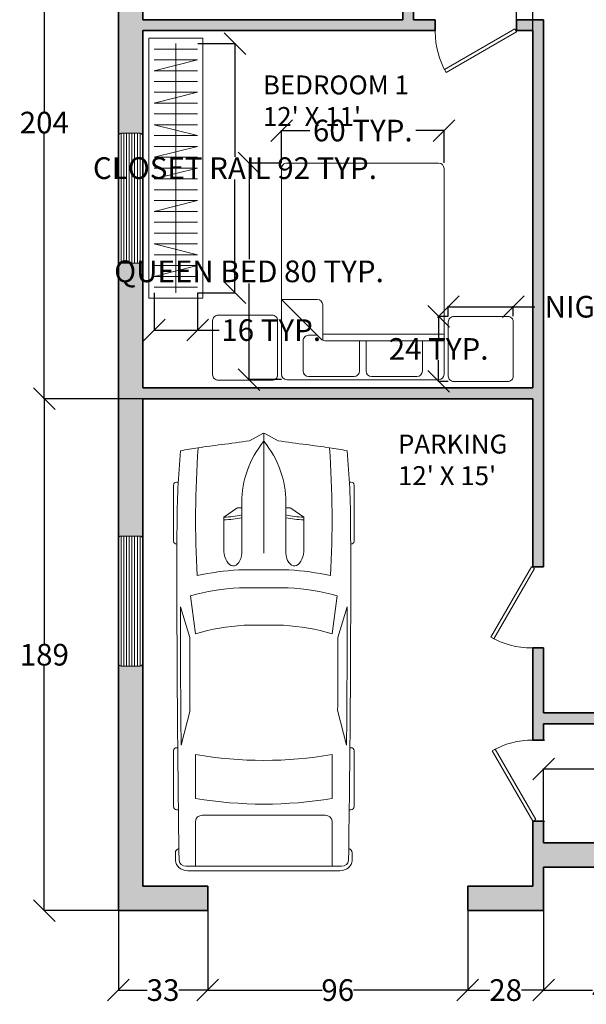
# Model space of a CAD drawing. Units: inches. Extents: x -8 to 447, y -560 to 47.
# Tile 1 of 5: x -8 to 201, y -560 to -196. Entities that reach past the tile are written whole.
import ezdxf

# ---------------------------------------------------------------- set-up
doc = ezdxf.new("R2010")
doc.units = ezdxf.units.IN
doc.header["$MEASUREMENT"] = 0
for name, color, linetype, lineweight in [('A-ANNO-DIMS', 2, 'Continuous', 18), ('A-AREA-IDEN', 7, 'Continuous', 18), ('A-FLOR-CASE', 8, 'Continuous', 18), ('A-FURN', 8, 'Continuous', 18), ('A-WALL', 7, 'Continuous', 35), ('A-WALL-PATT', 251, 'Continuous', 13), ('C-PKNG-VEHI', 8, 'Continuous', 13), ('DOOR', 40, 'Continuous', 18), ('WINDOW', 151, 'Continuous', 13)]:
    doc.layers.add(name, color=color, linetype=linetype, lineweight=lineweight)
doc.styles.get("Standard").update_dxf_attribs({"font": 'arial.ttf'})
doc.dimstyles.get("Standard").update_dxf_attribs({"dimtxt": 8, "dimasz": 8, "dimexe": 0.18, "dimexo": 0.0625, "dimgap": 0.09, "dimtad": 0, "dimtih": 1, "dimtoh": 1, "dimdec": 0, "dimzin": 0, "dimdsep": 46, "dimlunit": 4, "dimtxsty": 'Standard', "dimblk": 'OBLIQUE', "dimcen": 0.09, "dimadec": 0, "dimazin": 0, "dimtfac": 1, "dimtdec": 0, "dimtofl": 0, "dimtmove": 0, "dimatfit": 3, "dimldrblk": 'OBLIQUE', "dimfxl": 1, "dimtolj": 1, "dimtzin": 0, "dimarcsym": 0})

# ---------------------------------------------------------------- blocks, each defined once
blk = doc.blocks.new('WINDOW')
for p, q in [((0, -1.63), (48, -1.63)), ((0, -2.63), (48, -2.63)), ((0, -3.63), (48, -3.63)), ((0, -4.63), (48, -4.63)), ((0, -5.63), (48, -5.63)), ((0, -6.63), (48, -6.63)), ((0, -7.63), (48, -7.63)), ((0, -8.63), (48, -8.63))]:
    blk.add_line(p, q)
blk.add_lwpolyline([(48, -1.63), (48, -8.63, -0.414214), (47, -9.63), (1, -9.63, -0.414214), (0, -8.63), (0, -1.63, -0.414214), (1, -0.63), (47, -0.63, -0.414214)], format="xyb", close=True)
blk = doc.blocks.new('*U6')
for p, q in [((-40, 0), (-40, 6)), ((0, 0), (0, 6))]:
    blk.add_line(p, q)
blk.add_lwpolyline([(0, 0), (-34.64, -20), (-35.52, -18.48), (-0.88, 1.52)], close=True)
blk.add_arc((0, 0), 40, 180, 210)
blk = doc.blocks.new('*U4')
for p, q in [((0, 0), (0, 6)), ((40, 0), (40, 6))]:
    blk.add_line(p, q)
blk.add_lwpolyline([(0, 0), (34.64, -20), (35.52, -18.48), (0.87, 1.52)], close=True)
blk.add_arc((0, 0), 40, 330, 0)
blk = doc.blocks.new('Bed - Queen')
for p, q in [((2, 0), (58, 0)), ((0, -78), (0, -2)), ((8, -14.4), (8, -3.2)), ((10, -1.2), (26.8, -1.2)), ((28.8, -3.2), (28.8, -14.4)), ((31.2, -14.4), (31.2, -3.2)), ((33.2, -1.2), (50, -1.2)), ((52, -3.2), (52, -14.4)), ((60, -2), (60, -78)), ((0, -14.4), (43.97, -14.4)), ((44.8, -16.8), (0, -16.8)), ((44.8, -14.58), (44.8, -27.6)), ((60, -29.6), (45.39, -14.99)), ((50, -16.4), (46.8, -16.4)), ((46.8, -29.6), (60, -29.6)), ((58, -80), (2, -80))]:
    blk.add_line(p, q)
for centre, start, end in [((2, -2), 90, 180), ((58, -2), 0, 90), ((10, -3.2), 90, 180), ((26.8, -3.2), 0, 90), ((33.2, -3.2), 90, 180), ((50, -3.2), 0, 90), ((43.97, -16.4), 45, 90), ((50, -14.4), 270, 0), ((46.8, -27.6), 180, 270), ((2, -78), 180, 270), ((58, -78), 270, 0)]:
    blk.add_arc(centre, 2, start, end)
blk = doc.blocks.new('*U25')
for p, q in [((46.55, 38.89), (22.35, 38.89)), ((136.7, 38.89), (160.9, 38.89)), ((21.1, 37.41), (21.1, 36.83)), ((47.8, 37.39), (47.8, 37.41)), ((87.99, 31.87), (74.76, 35.92)), ((134.31, 35.6), (119.29, 31.78)), ((135.45, 37.07), (135.45, 37.41)), ((162.15, 37.41), (162.15, 36.77)), ((70.03, 31.54), (86.41, 29.35)), ((186.47, -33.5), (186.47, 33.5)), ((188.4, -32.76), (188.4, 32.76)), ((138.42, 29.35), (157.25, 29.35)), ((164.52, 26.39), (164.52, -26.39)), ((186.47, 29.35), (167.01, 29.35)), ((32.27, 11.63), (36.13, 17.17)), ((36.13, 17.17), (50.94, 17.17)), ((29.77, 9.51), (51.68, 9.51)), ((32.12, 9.51), (32.12, 11.15)), ((58.92, -10.77), (58.92, 10.77)), ((66.55, -10.53), (66.55, 10.53)), ((82.74, 8.5), (82.74, -8.5)), ((186.47, -10.53), (186.47, 10.53)), ((3.27, 6.13), (0.1, 0.41)), ((0, 0), (51.68, 0)), ((0.1, -0.41), (3.27, -6.13)), ((29.77, -9.51), (51.68, -9.51)), ((32.12, -9.51), (32.12, -11.15)), ((32.27, -11.63), (36.13, -17.17)), ((36.13, -17.17), (50.94, -17.17)), ((86.41, -29.35), (70.03, -31.54)), ((157.25, -29.35), (138.42, -29.35)), ((167.01, -29.35), (186.47, -29.35)), ((87.99, -31.87), (74.76, -35.92)), ((134.31, -35.6), (119.29, -31.78)), ((21.1, -37.41), (21.1, -36.83)), ((47.8, -37.39), (47.8, -37.41)), ((135.45, -37.07), (135.45, -37.41)), ((162.15, -37.41), (162.15, -36.77)), ((46.55, -38.89), (22.35, -38.89)), ((136.7, -38.89), (160.9, -38.89))]:
    blk.add_line(p, q)
for centre, major_axis, ratio, start_param, end_param in [((22.35, 37.41), (0, -1.48), 0.842304, 3.141593, 4.712389), ((46.55, 37.41), (0, 1.48), 0.842304, -1.570796, 0), ((136.7, 37.41), (0, -1.48), 0.842304, 3.141593, 4.712389), ((160.9, 37.41), (0, 1.48), 0.842304, -1.570796, 0), ((266.03, -27.52), (0, 313.31), 0.842304, 1.367076, 1.39176), ((41.19, -490.86), (0, 528.23), 0.842304, 0.00281, 0.075598), ((64.48, -10555.62), (0, 10593.03), 0.842304, -0.013397, 0.002797), ((64.48, -10555.62), (0, -10591.55), 0.842304, 3.133765, 3.140441), ((180.63, 35.84), (0, 2.22), 0.842304, -0.013017, 1.249894), ((64.48, -10556.36), (0, 10595.31), 0.842304, -0.013397, -0.013017), ((183.98, 33.5), (0, -2.96), 0.842304, 1.570796, 3.128196), ((183.98, 32.76), (0, -5.25), 0.842304, 1.570796, 3.128196), ((37.47, -593.96), (0, -623.33), 0.842304, 3.096046, 3.200911), ((135.29, 5.39), (0, 81.77), 0.842304, 1.245306, 1.50788), ((95.79, -3666.35), (0, -3698.24), 0.842304, 3.134049, 3.144098), ((259.18, -27.52), (0, -305.3), 0.842304, 4.528606, 4.561838), ((134.4, 5.39), (0, -89.78), 0.842304, 4.449482, 4.652344), ((149.6, 2.8), (0, -79.58), 0.842304, 4.372215, 4.640744), ((17.08, 0), (0, 147.02), 0.842304, 4.511394, 4.913384), ((35.91, 0), (0, 147.02), 0.842304, 4.511394, 4.913384), ((167.01, 26.39), (0, 2.96), 0.842304, 0, 1.570796), ((-204.49, 52.4), (0, -250.96), 0.842304, 1.385369, 1.434372), ((13.04, 17.01), (0, 27.42), 0.842304, 4.435146, 4.718221), ((14.2, 17.01), (0, 27.42), 0.842304, 4.435146, 4.718221), ((50.79, 13.34), (6.34, -0.36), 0.603834, -1.395552, 1.581315), ((29.77, -46.66), (0, 56.17), 0.842304, 0, 0.590319), ((32.75, 11.15), (0, 0.74), 0.842304, 0.879714, 1.570796), ((0.62, 0), (0, -0.74), 0.842304, 4.131459, 5.293319), ((29.77, 46.66), (0, 56.17), 0.842304, 2.551274, 3.141593), ((-204.49, -52.4), (0, 250.96), 0.842304, -1.434372, -1.385369), ((32.75, -11.15), (0, -0.74), 0.842304, 4.712389, 5.403472), ((13.04, -17.01), (0, -27.42), 0.842304, 1.564964, 1.848039), ((14.2, -17.01), (0, -27.42), 0.842304, 1.564964, 1.848039), ((134.4, -5.39), (0, -89.78), 0.842304, -1.510751, -1.307889), ((135.29, -5.39), (0, -81.77), 0.842304, -1.50788, -1.245306), ((149.6, -2.8), (0, -79.58), 0.842304, -1.499151, -1.230623), ((259.18, 27.52), (0, 305.3), 0.842304, 1.721348, 1.754579), ((266.03, 27.52), (0, 313.31), 0.842304, 1.749832, 1.774517), ((37.47, 593.96), (0, -623.33), 0.842304, -0.059319, 0.045547), ((167.01, -26.39), (0, -2.96), 0.842304, 4.712389, 6.283185), ((95.79, 3666.35), (0, -3698.24), 0.842304, -0.002505, 0.007544), ((183.98, -33.5), (0, 2.96), 0.842304, 3.15499, 4.712389), ((183.98, -32.76), (0, -5.25), 0.842304, 0.013397, 1.570796), ((41.19, 490.86), (0, -528.23), 0.842304, -0.075598, -0.00281), ((22.35, -37.41), (0, 1.48), 0.842304, 1.570796, 3.141593), ((64.48, 10555.62), (0, 10593.03), 0.842304, 3.138796, 3.15499), ((46.55, -37.41), (0, -1.48), 0.842304, 0, 1.570796), ((64.48, 10555.62), (0, -10591.55), 0.842304, 0.001152, 0.007828), ((136.7, -37.41), (0, -1.48), 0.842304, -1.570796, 0), ((160.9, -37.41), (0, 1.48), 0.842304, 3.141593, 4.712389), ((180.63, -35.84), (0, -2.22), 0.842304, -1.249894, 0.013017), ((64.48, 10556.36), (0, 10595.31), 0.842304, 3.15461, 3.15499)]:
    blk.add_ellipse(centre, major_axis=major_axis, ratio=ratio, start_param=start_param, end_param=end_param)
at = {"extrusion": (0, 0, -1)}
blk.add_ellipse((50.79, -13.34), major_axis=(6.34, 0.36), ratio=0.603834, start_param=-1.395552, end_param=1.581315, dxfattribs=at)
blk = doc.blocks.new('CLOSET-HANGING-RAIL-96IN')
for p, q in [((8, 0), (8, 92)), ((16, 90), (0, 90)), ((16, 86), (0, 86)), ((16, 86), (0, 82)), ((16, 82), (0, 82)), ((16, 78), (0, 78)), ((16, 74), (0, 74)), ((16, 74), (0, 70)), ((16, 70), (0, 70)), ((16, 66), (0, 66)), ((16, 62), (0, 62)), ((0, 62), (16, 58)), ((16, 58), (0, 58)), ((16, 54), (0, 54)), ((16, 54), (0, 50)), ((16, 50), (0, 50)), ((16, 46), (0, 46)), ((16, 46), (0, 42)), ((16, 42), (0, 42)), ((16, 38), (0, 38)), ((16, 34), (0, 34)), ((16, 34), (0, 30)), ((16, 30), (0, 30)), ((16, 26), (0, 26)), ((16, 22), (0, 22)), ((16, 18), (0, 18)), ((0, 18), (16, 14)), ((16, 14), (0, 14)), ((16, 10), (0, 10)), ((16, 10), (0, 6)), ((16, 6), (0, 6)), ((16, 2), (0, 2))]:
    blk.add_line(p, q)
blk = doc.blocks.new('NIGHTSTAND-24IN')
blk.add_lwpolyline([(22, 0), (2, 0, -0.414214), (0, 2), (0, 22, -0.414214), (2, 24), (22, 24, -0.414214), (24, 22), (24, 2, -0.414214)], format="xyb", close=True)
blk = doc.blocks.new('_Oblique')
at = {"color": 0, "linetype": 'ByBlock', "lineweight": -2}
blk.add_line((-0.5, -0.5), (0.5, 0.5), dxfattribs=at)
blk = doc.blocks.new('*D33')
at = {"layer": 'A-ANNO-DIMS', "color": 0, "lineweight": -2, "transparency": 16777216}
for p, q in [((150.53, -305.97), (150.53, -302.25)), ((150.53, -302.43), (174.53, -302.43)), ((174.53, -305.97), (174.53, -302.25)), ((174.53, -302.43), (182.53, -302.43))]:
    blk.add_line(p, q, dxfattribs=at)
at = {"layer": 'Defpoints', "color": 0, "transparency": 16777216}
for p in [(174.53, -302.43), (150.53, -306.03), (174.53, -306.03)]:
    blk.add_point(p, dxfattribs=at)
at = {"layer": 'A-ANNO-DIMS', "color": 0, "lineweight": -2, "transparency": 16777216, "xscale": 8, "yscale": 8, "zscale": 8, "rotation": 180}
blk.add_blockref('_Oblique', (150.53, -302.43), dxfattribs=at)
at = {"layer": 'A-ANNO-DIMS', "color": 0, "lineweight": -2, "transparency": 16777216, "xscale": 8, "yscale": 8, "zscale": 8}
blk.add_blockref('_Oblique', (174.53, -302.43), dxfattribs=at)
at = {"layer": 'A-ANNO-DIMS', "color": 0, "transparency": 16777216, "insert": (239.77, -302.43), "char_height": 8, "attachment_point": 5}
blk.add_mtext('\\A1;NIGHTSTAND 24 TYP.', dxfattribs=at)
blk = doc.blocks.new('*D34')
at = {"layer": 'A-ANNO-DIMS', "color": 0, "lineweight": -2, "transparency": 16777216}
for p, q in [((150.47, -306.03), (146.75, -306.03)), ((146.93, -306.03), (146.93, -313.92)), ((146.93, -330.03), (146.93, -322.14)), ((150.47, -330.03), (146.75, -330.03))]:
    blk.add_line(p, q, dxfattribs=at)
at = {"layer": 'Defpoints', "color": 0, "transparency": 16777216}
for p in [(146.93, -306.03), (150.53, -306.03), (150.53, -330.03)]:
    blk.add_point(p, dxfattribs=at)
at = {"layer": 'A-ANNO-DIMS', "color": 0, "lineweight": -2, "transparency": 16777216, "xscale": 8, "yscale": 8, "zscale": 8}
for p, rotation in [((146.93, -306.03), 90), ((146.93, -330.03), 270)]:
    blk.add_blockref('_Oblique', p, dxfattribs=dict(at, rotation=rotation))
at = {"layer": 'A-ANNO-DIMS', "color": 0, "transparency": 16777216, "insert": (146.93, -318.03), "char_height": 8, "attachment_point": 5}
blk.add_mtext('\\A1;24 TYP.', dxfattribs=at)
blk = doc.blocks.new('*D35')
at = {"layer": 'A-ANNO-DIMS', "color": 0, "lineweight": -2, "transparency": 16777216}
for p, q in [((88.88, -249.37), (76.76, -249.37)), ((76.94, -249.37), (76.94, -284.9)), ((76.94, -329.37), (76.94, -293.85)), ((88.88, -329.37), (76.76, -329.37))]:
    blk.add_line(p, q, dxfattribs=at)
at = {"layer": 'Defpoints', "color": 0, "transparency": 16777216}
for p in [(88.94, -249.37), (76.94, -329.37), (88.94, -329.37)]:
    blk.add_point(p, dxfattribs=at)
at = {"layer": 'A-ANNO-DIMS', "color": 0, "lineweight": -2, "transparency": 16777216, "xscale": 8, "yscale": 8, "zscale": 8}
for p, rotation in [((76.94, -249.37), 90), ((76.94, -329.37), 270)]:
    blk.add_blockref('_Oblique', p, dxfattribs=dict(at, rotation=rotation))
at = {"layer": 'A-ANNO-DIMS', "color": 0, "transparency": 16777216, "insert": (76.94, -289.37), "char_height": 8, "attachment_point": 5}
blk.add_mtext('\\A1;QUEEN BED 80 TYP.', dxfattribs=at)
blk = doc.blocks.new('*D36')
at = {"layer": 'A-ANNO-DIMS', "color": 0, "lineweight": -2, "transparency": 16777216}
for p, q in [((88.94, -249.31), (88.94, -237.19)), ((88.94, -237.37), (99.36, -237.37)), ((148.94, -237.37), (138.53, -237.37)), ((148.94, -249.31), (148.94, -237.19))]:
    blk.add_line(p, q, dxfattribs=at)
at = {"layer": 'Defpoints', "color": 0, "transparency": 16777216}
for p in [(88.94, -237.37), (88.94, -249.37), (148.94, -249.37)]:
    blk.add_point(p, dxfattribs=at)
at = {"layer": 'A-ANNO-DIMS', "color": 0, "lineweight": -2, "transparency": 16777216, "xscale": 8, "yscale": 8, "zscale": 8, "rotation": 180}
blk.add_blockref('_Oblique', (88.94, -237.37), dxfattribs=at)
at = {"layer": 'A-ANNO-DIMS', "color": 0, "lineweight": -2, "transparency": 16777216, "xscale": 8, "yscale": 8, "zscale": 8}
blk.add_blockref('_Oblique', (148.94, -237.37), dxfattribs=at)
at = {"layer": 'A-ANNO-DIMS', "color": 0, "transparency": 16777216, "insert": (118.94, -237.37), "char_height": 8, "attachment_point": 5}
blk.add_mtext('\\A1;60 TYP.', dxfattribs=at)
blk = doc.blocks.new('*D37')
at = {"layer": 'A-ANNO-DIMS', "color": 0, "lineweight": -2, "transparency": 16777216}
for p, q in [((58.01, -205.26), (71.93, -205.26)), ((71.75, -205.26), (71.75, -247.03)), ((71.75, -297.26), (71.75, -255.49)), ((58.01, -297.26), (71.93, -297.26))]:
    blk.add_line(p, q, dxfattribs=at)
at = {"layer": 'Defpoints', "color": 0, "transparency": 16777216}
for p in [(57.95, -205.26), (71.75, -205.26), (57.95, -297.26)]:
    blk.add_point(p, dxfattribs=at)
at = {"layer": 'A-ANNO-DIMS', "color": 0, "lineweight": -2, "transparency": 16777216, "xscale": 8, "yscale": 8, "zscale": 8}
for p, rotation in [((71.75, -205.26), 90), ((71.75, -297.26), 270)]:
    blk.add_blockref('_Oblique', p, dxfattribs=dict(at, rotation=rotation))
at = {"layer": 'A-ANNO-DIMS', "color": 0, "transparency": 16777216, "insert": (71.75, -251.26), "char_height": 8, "attachment_point": 5}
blk.add_mtext('\\A1;CLOSET RAIL 92 TYP.', dxfattribs=at)
blk = doc.blocks.new('*D38')
at = {"layer": 'A-ANNO-DIMS', "color": 0, "lineweight": -2, "transparency": 16777216}
for p, q in [((41.95, -297.33), (41.95, -311.24)), ((57.95, -297.33), (57.95, -311.24)), ((41.95, -311.06), (57.95, -311.06)), ((57.95, -311.06), (65.95, -311.06))]:
    blk.add_line(p, q, dxfattribs=at)
at = {"layer": 'Defpoints', "color": 0, "transparency": 16777216}
for p in [(41.95, -297.26), (57.95, -297.26), (57.95, -311.06)]:
    blk.add_point(p, dxfattribs=at)
at = {"layer": 'A-ANNO-DIMS', "color": 0, "lineweight": -2, "transparency": 16777216, "xscale": 8, "yscale": 8, "zscale": 8, "rotation": 180}
blk.add_blockref('_Oblique', (41.95, -311.06), dxfattribs=at)
at = {"layer": 'A-ANNO-DIMS', "color": 0, "lineweight": -2, "transparency": 16777216, "xscale": 8, "yscale": 8, "zscale": 8}
blk.add_blockref('_Oblique', (57.95, -311.06), dxfattribs=at)
at = {"layer": 'A-ANNO-DIMS', "color": 0, "transparency": 16777216, "insert": (85.13, -311.06), "char_height": 8, "attachment_point": 5}
blk.add_mtext('\\A1;16 TYP.', dxfattribs=at)
blk = doc.blocks.new('*D54')
at = {"layer": 'A-ANNO-DIMS', "color": 0, "lineweight": -2, "transparency": 16777216}
for p, q in [((37.64, -132.44), (1.17, -132.44)), ((1.35, -132.44), (1.35, -230.27)), ((1.35, -336.44), (1.35, -238.61)), ((37.64, -336.44), (1.17, -336.44))]:
    blk.add_line(p, q, dxfattribs=at)
at = {"layer": 'Defpoints', "color": 0, "transparency": 16777216}
for p in [(37.7, -132.44), (1.35, -336.44), (37.7, -336.44)]:
    blk.add_point(p, dxfattribs=at)
at = {"layer": 'A-ANNO-DIMS', "color": 0, "lineweight": -2, "transparency": 16777216, "xscale": 8, "yscale": 8, "zscale": 8}
for p, rotation in [((1.35, -132.44), 90), ((1.35, -336.44), 270)]:
    blk.add_blockref('_Oblique', p, dxfattribs=dict(at, rotation=rotation))
at = {"layer": 'A-ANNO-DIMS', "color": 0, "transparency": 16777216, "insert": (1.35, -234.44), "char_height": 8, "attachment_point": 5}
blk.add_mtext('\\A1;204', dxfattribs=at)
blk = doc.blocks.new('*D55')
at = {"layer": 'A-ANNO-DIMS', "color": 0, "lineweight": -2, "transparency": 16777216}
for p, q in [((37.64, -336.44), (1.17, -336.44)), ((1.35, -336.44), (1.35, -426.77)), ((1.35, -525.44), (1.35, -435.11)), ((28.64, -525.44), (1.17, -525.44))]:
    blk.add_line(p, q, dxfattribs=at)
at = {"layer": 'Defpoints', "color": 0, "transparency": 16777216}
for p in [(37.7, -336.44), (1.35, -525.44), (28.7, -525.44)]:
    blk.add_point(p, dxfattribs=at)
at = {"layer": 'A-ANNO-DIMS', "color": 0, "lineweight": -2, "transparency": 16777216, "xscale": 8, "yscale": 8, "zscale": 8}
for p, rotation in [((1.35, -336.44), 90), ((1.35, -525.44), 270)]:
    blk.add_blockref('_Oblique', p, dxfattribs=dict(at, rotation=rotation))
at = {"layer": 'A-ANNO-DIMS', "color": 0, "transparency": 16777216, "insert": (1.35, -430.94), "char_height": 8, "attachment_point": 5}
blk.add_mtext('\\A1;189', dxfattribs=at)
blk = doc.blocks.new('*D56')
at = {"layer": 'A-ANNO-DIMS', "color": 0, "lineweight": -2, "transparency": 16777216}
for p, q in [((28.7, -525.5), (28.7, -554.97)), ((61.7, -525.5), (61.7, -554.97)), ((28.7, -554.79), (39.39, -554.79)), ((61.7, -554.79), (51.02, -554.79))]:
    blk.add_line(p, q, dxfattribs=at)
at = {"layer": 'Defpoints', "color": 0, "transparency": 16777216}
for p in [(28.7, -525.44), (61.7, -525.44), (61.7, -554.79)]:
    blk.add_point(p, dxfattribs=at)
at = {"layer": 'A-ANNO-DIMS', "color": 0, "lineweight": -2, "transparency": 16777216, "xscale": 8, "yscale": 8, "zscale": 8, "rotation": 180}
blk.add_blockref('_Oblique', (28.7, -554.79), dxfattribs=at)
at = {"layer": 'A-ANNO-DIMS', "color": 0, "lineweight": -2, "transparency": 16777216, "xscale": 8, "yscale": 8, "zscale": 8}
blk.add_blockref('_Oblique', (61.7, -554.79), dxfattribs=at)
at = {"layer": 'A-ANNO-DIMS', "color": 0, "transparency": 16777216, "insert": (45.2, -554.79), "char_height": 8, "attachment_point": 5}
blk.add_mtext('\\A1;33', dxfattribs=at)
blk = doc.blocks.new('*D57')
at = {"layer": 'A-ANNO-DIMS', "color": 0, "lineweight": -2, "transparency": 16777216}
for p, q in [((61.7, -525.5), (61.7, -554.97)), ((157.7, -525.5), (157.7, -554.97)), ((61.7, -554.79), (103.89, -554.79)), ((157.7, -554.79), (115.52, -554.79))]:
    blk.add_line(p, q, dxfattribs=at)
at = {"layer": 'Defpoints', "color": 0, "transparency": 16777216}
for p in [(61.7, -525.44), (157.7, -525.44), (157.7, -554.79)]:
    blk.add_point(p, dxfattribs=at)
at = {"layer": 'A-ANNO-DIMS', "color": 0, "lineweight": -2, "transparency": 16777216, "xscale": 8, "yscale": 8, "zscale": 8, "rotation": 180}
blk.add_blockref('_Oblique', (61.7, -554.79), dxfattribs=at)
at = {"layer": 'A-ANNO-DIMS', "color": 0, "lineweight": -2, "transparency": 16777216, "xscale": 8, "yscale": 8, "zscale": 8}
blk.add_blockref('_Oblique', (157.7, -554.79), dxfattribs=at)
at = {"layer": 'A-ANNO-DIMS', "color": 0, "transparency": 16777216, "insert": (109.7, -554.79), "char_height": 8, "attachment_point": 5}
blk.add_mtext('\\A1;96', dxfattribs=at)
blk = doc.blocks.new('*D58')
at = {"layer": 'A-ANNO-DIMS', "color": 0, "lineweight": -2, "transparency": 16777216}
for p, q in [((157.7, -525.5), (157.7, -554.97)), ((185.7, -525.5), (185.7, -554.97)), ((157.7, -554.79), (165.81, -554.79)), ((185.7, -554.79), (177.6, -554.79))]:
    blk.add_line(p, q, dxfattribs=at)
at = {"layer": 'Defpoints', "color": 0, "transparency": 16777216}
for p in [(157.7, -525.44), (185.7, -525.44), (185.7, -554.79)]:
    blk.add_point(p, dxfattribs=at)
at = {"layer": 'A-ANNO-DIMS', "color": 0, "lineweight": -2, "transparency": 16777216, "xscale": 8, "yscale": 8, "zscale": 8, "rotation": 180}
blk.add_blockref('_Oblique', (157.7, -554.79), dxfattribs=at)
at = {"layer": 'A-ANNO-DIMS', "color": 0, "lineweight": -2, "transparency": 16777216, "xscale": 8, "yscale": 8, "zscale": 8}
blk.add_blockref('_Oblique', (185.7, -554.79), dxfattribs=at)
at = {"layer": 'A-ANNO-DIMS', "color": 0, "transparency": 16777216, "insert": (171.7, -554.79), "char_height": 8, "attachment_point": 5}
blk.add_mtext('\\A1;28', dxfattribs=at)
blk = doc.blocks.new('*D59')
at = {"layer": 'A-ANNO-DIMS', "color": 0, "lineweight": -2, "transparency": 16777216}
for p, q in [((233.7, -509.5), (233.7, -554.97)), ((185.7, -525.5), (185.7, -554.97)), ((185.7, -554.79), (203.71, -554.79)), ((233.7, -554.79), (215.69, -554.79))]:
    blk.add_line(p, q, dxfattribs=at)
at = {"layer": 'Defpoints', "color": 0, "transparency": 16777216}
for p in [(233.7, -509.44), (185.7, -525.44), (233.7, -554.79)]:
    blk.add_point(p, dxfattribs=at)
at = {"layer": 'A-ANNO-DIMS', "color": 0, "lineweight": -2, "transparency": 16777216, "xscale": 8, "yscale": 8, "zscale": 8, "rotation": 180}
blk.add_blockref('_Oblique', (185.7, -554.79), dxfattribs=at)
at = {"layer": 'A-ANNO-DIMS', "color": 0, "lineweight": -2, "transparency": 16777216, "xscale": 8, "yscale": 8, "zscale": 8}
blk.add_blockref('_Oblique', (233.7, -554.79), dxfattribs=at)
at = {"layer": 'A-ANNO-DIMS', "color": 0, "transparency": 16777216, "insert": (209.7, -554.79), "char_height": 8, "attachment_point": 5}
blk.add_mtext('\\A1;48', dxfattribs=at)
blk = doc.blocks.new('*D64')
at = {"layer": 'A-ANNO-DIMS', "color": 0, "lineweight": -2, "transparency": 16777216}
for p, q in [((185.7, -500.38), (185.7, -472.91)), ((185.7, -473.09), (269.17, -473.09)), ((369.7, -473.09), (286.24, -473.09)), ((369.7, -500.38), (369.7, -472.91))]:
    blk.add_line(p, q, dxfattribs=at)
at = {"layer": 'Defpoints', "color": 0, "transparency": 16777216}
for p in [(369.7, -473.09), (185.7, -500.44), (369.7, -500.44)]:
    blk.add_point(p, dxfattribs=at)
at = {"layer": 'A-ANNO-DIMS', "color": 0, "lineweight": -2, "transparency": 16777216, "xscale": 8, "yscale": 8, "zscale": 8, "rotation": 180}
blk.add_blockref('_Oblique', (185.7, -473.09), dxfattribs=at)
at = {"layer": 'A-ANNO-DIMS', "color": 0, "lineweight": -2, "transparency": 16777216, "xscale": 8, "yscale": 8, "zscale": 8}
blk.add_blockref('_Oblique', (369.7, -473.09), dxfattribs=at)
at = {"layer": 'A-ANNO-DIMS', "color": 0, "transparency": 16777216, "insert": (277.7, -473.09), "char_height": 8, "attachment_point": 5}
blk.add_mtext('\\A1;184', dxfattribs=at)
blk = doc.blocks.new('*D65')
at = {"layer": 'A-ANNO-DIMS', "color": 0, "lineweight": -2, "transparency": 16777216}
for p, q in [((185.764836, -456.440047), (213.232336, -456.440047)), ((213.052336, -456.440047), (213.052336, -474.350047)), ((213.052336, -500.440047), (213.052336, -482.530047)), ((185.764836, -500.440047), (213.232336, -500.440047))]:
    blk.add_line(p, q, dxfattribs=at)
at = {"layer": 'Defpoints', "color": 0, "transparency": 16777216}
for p in [(185.702336, -456.440047), (185.702336, -500.440047), (213.052336, -500.440047)]:
    blk.add_point(p, dxfattribs=at)
at = {"layer": 'A-ANNO-DIMS', "color": 0, "lineweight": -2, "transparency": 16777216, "xscale": 8, "yscale": 8, "zscale": 8}
for p, rotation in [((213.052336, -456.440047), 90), ((213.052336, -500.440047), 270)]:
    blk.add_blockref('_Oblique', p, dxfattribs=dict(at, rotation=rotation))
at = {"layer": 'A-ANNO-DIMS', "color": 0, "transparency": 16777216, "insert": (213.052336, -478.440047), "char_height": 8, "attachment_point": 5}
blk.add_mtext('\\A1;44', dxfattribs=at)
blk = doc.blocks.new('*D69')
at = {"layer": 'A-ANNO-DIMS', "color": 0, "lineweight": -2, "transparency": 16777216}
for p, q in [((175.7, -200.38), (175.7, 42.09)), ((175.7, 41.91), (175.97, 41.91)), ((181.7, 41.91), (181.43, 41.91)), ((181.7, -200.38), (181.7, 42.09))]:
    blk.add_line(p, q, dxfattribs=at)
at = {"layer": 'Defpoints', "color": 0, "transparency": 16777216}
for p in [(181.7, 41.91), (175.7, -200.44), (181.7, -200.44)]:
    blk.add_point(p, dxfattribs=at)
at = {"layer": 'A-ANNO-DIMS', "color": 0, "lineweight": -2, "transparency": 16777216, "xscale": 8, "yscale": 8, "zscale": 8, "rotation": 180}
blk.add_blockref('_Oblique', (175.7, 41.91), dxfattribs=at)
at = {"layer": 'A-ANNO-DIMS', "color": 0, "lineweight": -2, "transparency": 16777216, "xscale": 8, "yscale": 8, "zscale": 8}
blk.add_blockref('_Oblique', (181.7, 41.91), dxfattribs=at)
at = {"layer": 'A-ANNO-DIMS', "color": 0, "transparency": 16777216, "insert": (178.7, 41.91), "char_height": 8, "attachment_point": 5}
blk.add_mtext('\\A1;6', dxfattribs=at)

msp = doc.modelspace()

# ---------------------------------------------------------------- hatches: boundary and pattern name
at = {"layer": 'A-WALL-PATT'}
h = msp.add_hatch(color=256, dxfattribs=at)
h.dxf.hatch_style = 1
h.paths.add_polyline_path([(37.702, -178.44), (28.702, -178.44), (28.702, -238.368), (37.702, -238.368), (37.702, -200.44), (145.702, -200.44), (145.702, -196.44), (137.702, -196.44), (137.702, -172.44), (133.702, -172.44), (133.702, -196.44), (37.702, -196.44)])
h = msp.add_hatch(color=256, dxfattribs=at)
h.dxf.hatch_style = 1
h.paths.add_polyline_path([(185.702, -196.44), (175.702, -196.44), (175.702, -200.44), (181.702, -200.44), (181.702, -332.44), (37.702, -332.44), (37.702, -286.368), (28.702, -286.368), (28.702, -387.116), (37.702, -387.116), (37.702, -336.44), (181.702, -336.44), (181.702, -398.44), (185.702, -398.44)])
h = msp.add_hatch(color=256, dxfattribs=at)
h.dxf.hatch_style = 1
h.paths.add_polyline_path([(37.702, -286.368), (28.702, -286.368), (28.702, -387.116), (37.702, -387.116), (37.702, -336.44), (181.702, -336.44), (181.702, -332.44), (37.702, -332.44)])
h = msp.add_hatch(color=256, dxfattribs=at)
h.dxf.hatch_style = 1
h.paths.add_polyline_path([(61.702, -516.44), (37.702, -516.44), (37.702, -435.116), (28.702, -435.116), (28.702, -525.44), (61.702, -525.44)])
h.paths.add_polyline_path([(185.702, -509.44), (233.702, -509.44), (233.702, -500.44), (185.702, -500.44), (185.702, -492.44), (181.702, -492.44), (181.702, -516.44), (157.702, -516.44), (157.702, -525.44), (185.702, -525.44)])
h.paths.add_polyline_path([(229.702, -452.44), (185.702, -452.44), (185.702, -428.44), (181.702, -428.44), (181.702, -462.44), (185.702, -462.44), (185.702, -456.44), (229.702, -456.44)])

# ---------------------------------------------------------------- linework, layer by layer
at = {"layer": 'A-FLOR-CASE'}
for p, q in [((59.947, -203.264), (39.947, -203.264)), ((39.947, -203.264), (39.947, -299.264)), ((59.947, -299.264), (59.947, -203.264)), ((39.947, -299.264), (59.947, -299.264)), ((59.947, -299.264), (39.947, -299.264))]:
    msp.add_line(p, q, dxfattribs=at)
at = {"layer": 'A-WALL'}
for p, q in [((28.702, -525.44), (28.702, 14.56)), ((37.702, -196.44), (37.702, -136.44)), ((133.702, -196.44), (133.702, -172.44)), ((137.702, -196.44), (137.702, -172.44)), ((133.702, -196.44), (37.702, -196.44)), ((145.702, -196.44), (137.702, -196.44)), ((145.702, -200.44), (145.702, -196.44)), ((185.702, -196.44), (175.702, -196.44)), ((175.702, -200.44), (175.702, -196.44)), ((185.702, -398.44), (185.702, -196.44)), ((145.702, -200.44), (37.702, -200.44)), ((37.702, -332.44), (37.702, -200.44)), ((181.702, -200.44), (175.702, -200.44)), ((181.702, -332.44), (181.702, -200.44)), ((181.702, -332.44), (37.702, -332.44)), ((37.702, -516.44), (37.702, -336.44)), ((181.702, -336.44), (37.702, -336.44)), ((181.702, -398.44), (181.702, -336.44)), ((185.702, -398.44), (181.702, -398.44)), ((185.702, -428.44), (181.702, -428.44)), ((181.702, -462.44), (181.702, -428.44)), ((185.702, -452.44), (185.702, -428.44)), ((229.702, -452.44), (185.702, -452.44)), ((185.702, -462.44), (185.702, -456.44)), ((229.702, -456.44), (185.702, -456.44)), ((185.702, -462.44), (181.702, -462.44)), ((181.702, -516.44), (181.702, -492.44)), ((185.702, -492.44), (181.702, -492.44)), ((185.702, -500.44), (185.702, -492.44)), ((185.702, -500.44), (233.702, -500.44)), ((185.702, -525.44), (185.702, -509.44)), ((233.702, -509.44), (185.702, -509.44)), ((61.702, -516.44), (37.702, -516.44)), ((61.702, -516.44), (61.702, -525.44)), ((181.702, -516.44), (157.702, -516.44)), ((157.702, -516.44), (157.702, -525.44)), ((61.702, -525.44), (28.702, -525.44)), ((185.702, -525.44), (157.702, -525.44))]:
    msp.add_line(p, q, dxfattribs=at)

# ---------------------------------------------------------------- block references
at = {"layer": 'A-FLOR-CASE'}
msp.add_blockref('CLOSET-HANGING-RAIL-96IN', (41.947, -297.264), dxfattribs=at)
at = {"layer": 'A-FURN', "rotation": 180}
msp.add_blockref('Bed - Queen', (148.945, -329.375), dxfattribs=at)
at = {"layer": 'A-FURN'}
for p in [(63.514, -329.56), (150.53, -330.03)]:
    msp.add_blockref('NIGHTSTAND-24IN', p, dxfattribs=at)
at = {"layer": 'C-PKNG-VEHI', "xscale": 0.8576856779474988, "yscale": 0.8576856779474988, "zscale": 0.8576856779474988, "rotation": 270}
msp.add_blockref('*U25', (82.406, -349.108), dxfattribs=at)
at = {"layer": 'DOOR', "xscale": 0.75, "yscale": 0.75, "zscale": 0.75}
msp.add_blockref('*U6', (175.702, -200.94), dxfattribs=at)
at = {"layer": 'DOOR', "xscale": 0.75, "yscale": 0.75, "zscale": 0.75, "rotation": 270}
for name, p in [('*U4', (181.202, -398.44)), ('*U6', (181.702, -492.44))]:
    msp.add_blockref(name, p, dxfattribs=at)
at = {"layer": 'WINDOW', "rotation": 270}
for p in [(38.337, -238.368), (38.337, -387.116)]:
    msp.add_blockref('WINDOW', p, dxfattribs=at)

# ---------------------------------------------------------------- texts
at = {"layer": 'A-AREA-IDEN', "char_height": 7, "attachment_point": 1}
for s, width, insert in [("BEDROOM 1 \\P12' X 11'", 129.75324, (82.07, -217.033)), ("PARKING \\P12' X 15'", 134.75943, (131.948, -349.652))]:
    msp.add_mtext_dynamic_manual_height_columns(s, width=width, gutter_width=1, heights=[0], dxfattribs=dict(at, insert=insert))

# ---------------------------------------------------------------- dimensions: what is measured, and where the dimension line sits
at = {"layer": 'A-ANNO-DIMS'}
for base, p1, p2, picture, middle in [((181.702, 41.91), (175.702, -200.44), (181.702, -200.44), '*D69', (178.702, 41.91)), ((369.702, -473.09), (185.702, -500.44), (369.702, -500.44), '*D64', (277.702, -473.09)), ((233.702, -554.79), (185.702, -525.44), (233.702, -509.44), '*D59', (209.702, -554.79)), ((61.702, -554.79), (28.702, -525.44), (61.702, -525.44), '*D56', (45.202, -554.79)), ((157.702, -554.79), (61.702, -525.44), (157.702, -525.44), '*D57', (109.702, -554.79)), ((185.702, -554.79), (157.702, -525.44), (185.702, -525.44), '*D58', (171.702, -554.79))]:
    dim = msp.add_linear_dim(base=base, p1=p1, p2=p2, dimstyle='Standard', override={"dimdec": 0, "dimlfac": 1, "dimrnd": 0, "dimzin": 0, "dimdsep": 46, "dimlunit": 2}, dxfattribs=at)
    dim.commit()
    dim.dimension.update_dxf_attribs({"geometry": picture, "text_midpoint": middle})
for base, p1, p2, angle, picture, middle in [((1.352, -336.44), (37.702, -132.44), (37.702, -336.44), 90, '*D54', (1.352, -234.44)), ((1.352, -525.44), (37.702, -336.44), (28.702, -525.44), 90, '*D55', (1.352, -430.94)), ((213.052, -500.44), (185.702, -456.44), (185.702, -500.44), 270, '*D65', (213.052, -478.44))]:
    dim = msp.add_linear_dim(base=base, p1=p1, p2=p2, angle=angle, dimstyle='Standard', override={"dimdec": 0, "dimlfac": 1, "dimrnd": 0, "dimzin": 0, "dimdsep": 46, "dimlunit": 2}, dxfattribs=at)
    dim.commit()
    dim.dimension.update_dxf_attribs({"geometry": picture, "text_midpoint": middle})
for base, p1, p2, angle, text, picture, middle in [((71.747, -205.264), (57.947, -297.264), (57.947, -205.264), 90, 'CLOSET RAIL <> TYP.', '*D37', (71.747, -251.264)), ((88.945, -237.375), (148.945, -249.375), (88.945, -249.375), 180, '<> TYP.', '*D36', (118.945, -237.375)), ((76.945, -329.375), (88.945, -249.375), (88.945, -329.375), 270, 'QUEEN BED <> TYP.', '*D35', (76.945, -289.375)), ((146.93, -306.031), (150.53, -330.031), (150.53, -306.031), 90, '<> TYP.', '*D34', (146.93, -318.031))]:
    dim = msp.add_linear_dim(base=base, p1=p1, p2=p2, angle=angle, text=text, dimstyle='Standard', override={"dimdec": 0, "dimlfac": 1, "dimrnd": 0, "dimzin": 0, "dimdsep": 46, "dimlunit": 2}, dxfattribs=at)
    dim.commit()
    dim.dimension.update_dxf_attribs({"geometry": picture, "text_midpoint": middle})
for base, p1, p2, text, picture, middle in [((174.53, -302.431), (150.53, -306.031), (174.53, -306.031), 'NIGHTSTAND <> TYP.', '*D33', (239.771, -302.431)), ((57.947, -311.064), (41.947, -297.264), (57.947, -297.264), '<> TYP.', '*D38', (85.131, -311.064))]:
    dim = msp.add_linear_dim(base=base, p1=p1, p2=p2, text=text, dimstyle='Standard', override={"dimdec": 0, "dimlfac": 1, "dimrnd": 0, "dimzin": 0, "dimdsep": 46, "dimlunit": 2}, dxfattribs=at)
    dim.commit()
    dim.dimension.update_dxf_attribs({"geometry": picture, "text_midpoint": middle})

doc.saveas('drawing.dxf')
